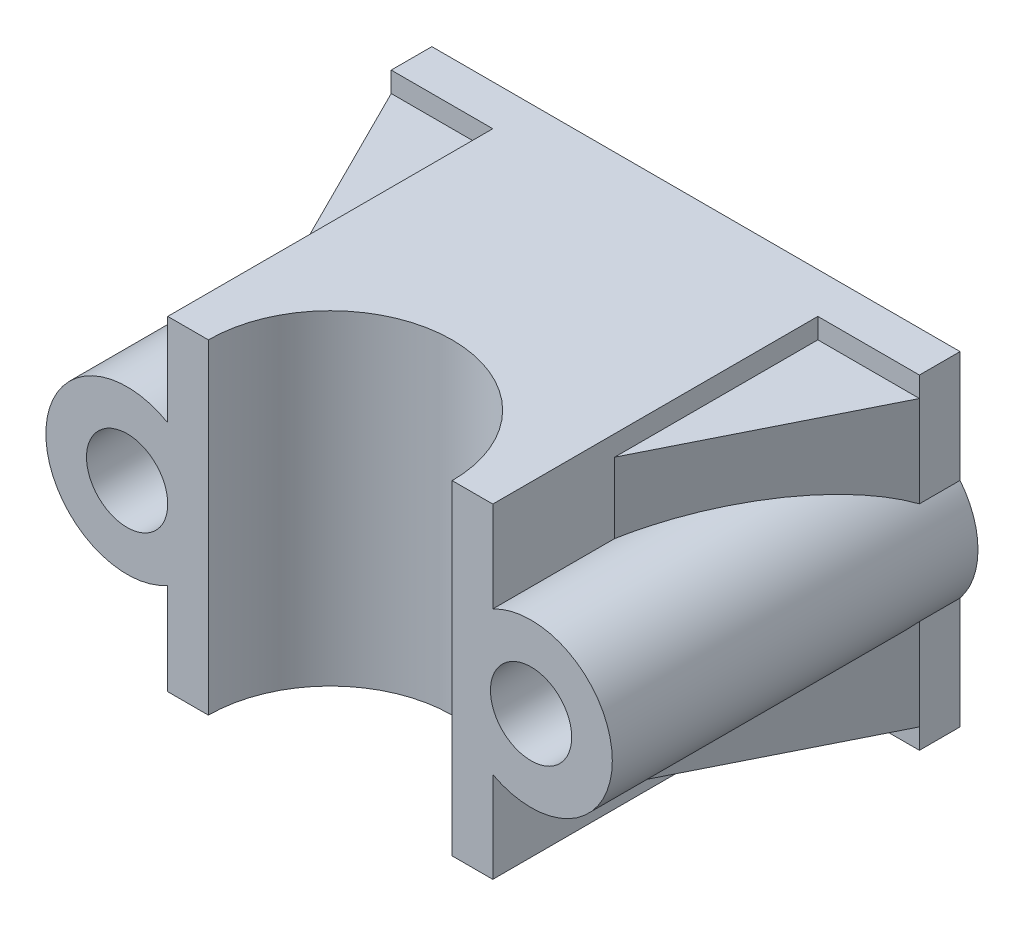
ISO-10303-21;
HEADER;
FILE_DESCRIPTION(('STEP AP214'),'2;1');
FILE_NAME('part.step','',(''),(''),'','','');
FILE_SCHEMA(('AUTOMOTIVE_DESIGN { 1 0 10303 214 1 1 1 1 }'));
ENDSEC;
DATA;
#1=APPLICATION_CONTEXT('core data for automotive mechanical design processes');
#2=APPLICATION_PROTOCOL_DEFINITION('international standard','automotive_design',2000,#1);
#3=PRODUCT_CONTEXT('',#1,'mechanical');
#4=PRODUCT('Part','Part','',(#3));
#5=PRODUCT_RELATED_PRODUCT_CATEGORY('part','',(#4));
#6=PRODUCT_DEFINITION_FORMATION('','',#4);
#7=PRODUCT_DEFINITION_CONTEXT('part definition',#1,'design');
#8=PRODUCT_DEFINITION('design','',#6,#7);
#9=PRODUCT_DEFINITION_SHAPE('','',#8);
#10=(LENGTH_UNIT() NAMED_UNIT(*) SI_UNIT(.MILLI.,.METRE.));
#11=(NAMED_UNIT(*) PLANE_ANGLE_UNIT() SI_UNIT($,.RADIAN.));
#12=(NAMED_UNIT(*) SI_UNIT($,.STERADIAN.) SOLID_ANGLE_UNIT());
#13=UNCERTAINTY_MEASURE_WITH_UNIT(LENGTH_MEASURE(1.E-05),#10,'distance_accuracy_value','');
#14=(GEOMETRIC_REPRESENTATION_CONTEXT(3) GLOBAL_UNCERTAINTY_ASSIGNED_CONTEXT((#13)) GLOBAL_UNIT_ASSIGNED_CONTEXT((#10,
#11,#12)) REPRESENTATION_CONTEXT('',''));
#15=CARTESIAN_POINT('',(0.,0.,0.));
#16=DIRECTION('',(0.,0.,1.));
#17=DIRECTION('',(1.,0.,0.));
#18=AXIS2_PLACEMENT_3D('',#15,#16,#17);
#19=CARTESIAN_POINT('',(105.,52.,60.));
#20=DIRECTION('',(0.894427190999916,0.,0.447213595499958));
#21=DIRECTION('',(0.447213595499958,0.,-0.894427190999916));
#22=AXIS2_PLACEMENT_3D('',#19,#20,#21);
#23=PLANE('',#22);
#24=DIRECTION('',(0.,1.,0.));
#25=VECTOR('',#24,1.);
#26=CARTESIAN_POINT('',(130.,0.,10.));
#27=LINE('',#26,#25);
#28=CARTESIAN_POINT('',(130.,52.5387472375144,10.));
#29=VERTEX_POINT('',#28);
#30=CARTESIAN_POINT('',(130.,75.,10.));
#31=VERTEX_POINT('',#30);
#32=EDGE_CURVE('E316',#29,#31,#27,.T.);
#33=ORIENTED_EDGE('',*,*,#32,.T.);
#34=DIRECTION('',(0.447213595499958,0.,-0.894427190999916));
#35=VECTOR('',#34,1.);
#36=CARTESIAN_POINT('',(130.,75.,10.));
#37=LINE('',#36,#35);
#38=CARTESIAN_POINT('',(105.,75.,60.));
#39=VERTEX_POINT('',#38);
#40=EDGE_CURVE('E420',#39,#31,#37,.T.);
#41=ORIENTED_EDGE('',*,*,#40,.F.);
#42=DIRECTION('',(0.,1.,0.));
#43=VECTOR('',#42,1.);
#44=CARTESIAN_POINT('',(105.,52.,60.));
#45=LINE('',#44,#43);
#46=CARTESIAN_POINT('',(105.,57.6434080653318,60.));
#47=VERTEX_POINT('',#46);
#48=EDGE_CURVE('E227',#47,#39,#45,.T.);
#49=ORIENTED_EDGE('',*,*,#48,.F.);
#50=CARTESIAN_POINT('',(114.418606682529,40.,41.1627866349416));
#51=DIRECTION('',(0.894427190999916,0.,0.447213595499958));
#52=DIRECTION('',(-0.447213595499958,0.,0.894427190999916));
#53=AXIS2_PLACEMENT_3D('',#50,#51,#52);
#54=ELLIPSE('',#53,44.7213595499958,20.);
#55=EDGE_CURVE('E54',#47,#29,#54,.F.);
#56=ORIENTED_EDGE('',*,*,#55,.T.);
#57=EDGE_LOOP('',(#33,#41,#49,#56));
#58=FACE_BOUND('',#57,.T.);
#59=ADVANCED_FACE('F50',(#58),#23,.T.);
#60=CARTESIAN_POINT('',(25.,28.,60.));
#61=DIRECTION('',(-0.894427190999916,0.,0.447213595499958));
#62=DIRECTION('',(0.447213595499958,0.,0.894427190999916));
#63=AXIS2_PLACEMENT_3D('',#60,#61,#62);
#64=PLANE('',#63);
#65=DIRECTION('',(0.,-1.,0.));
#66=VECTOR('',#65,1.);
#67=CARTESIAN_POINT('',(0.,80.,10.));
#68=LINE('',#67,#66);
#69=CARTESIAN_POINT('',(0.,26.771243444677,10.));
#70=VERTEX_POINT('',#69);
#71=CARTESIAN_POINT('',(0.,5.,10.));
#72=VERTEX_POINT('',#71);
#73=EDGE_CURVE('E324',#70,#72,#68,.T.);
#74=ORIENTED_EDGE('',*,*,#73,.T.);
#75=DIRECTION('',(-0.447213595499958,0.,-0.894427190999916));
#76=VECTOR('',#75,1.);
#77=CARTESIAN_POINT('',(0.,5.,10.));
#78=LINE('',#77,#76);
#79=CARTESIAN_POINT('',(25.,5.,60.));
#80=VERTEX_POINT('',#79);
#81=EDGE_CURVE('E426',#80,#72,#78,.T.);
#82=ORIENTED_EDGE('',*,*,#81,.F.);
#83=DIRECTION('',(0.,-1.,0.));
#84=VECTOR('',#83,1.);
#85=CARTESIAN_POINT('',(25.,28.,60.));
#86=LINE('',#85,#84);
#87=CARTESIAN_POINT('',(25.,22.6794919243112,60.));
#88=VERTEX_POINT('',#87);
#89=EDGE_CURVE('E233',#88,#80,#86,.T.);
#90=ORIENTED_EDGE('',*,*,#89,.F.);
#91=CARTESIAN_POINT('',(15.,40.,40.));
#92=DIRECTION('',(-0.894427190999916,0.,0.447213595499958));
#93=DIRECTION('',(0.447213595499958,0.,0.894427190999916));
#94=AXIS2_PLACEMENT_3D('',#91,#92,#93);
#95=ELLIPSE('',#94,44.7213595499958,20.);
#96=EDGE_CURVE('E359',#88,#70,#95,.F.);
#97=ORIENTED_EDGE('',*,*,#96,.T.);
#98=EDGE_LOOP('',(#74,#82,#90,#97));
#99=FACE_BOUND('',#98,.T.);
#100=ADVANCED_FACE('F466',(#99),#64,.T.);
#101=CARTESIAN_POINT('',(0.,80.,10.));
#102=DIRECTION('',(1.,0.,0.));
#103=DIRECTION('',(0.,0.,-1.));
#104=AXIS2_PLACEMENT_3D('',#101,#102,#103);
#105=PLANE('',#104);
#106=DIRECTION('',(0.,-1.,0.));
#107=VECTOR('',#106,1.);
#108=CARTESIAN_POINT('',(0.,80.,0.));
#109=LINE('',#108,#107);
#110=CARTESIAN_POINT('',(0.,80.,0.));
#111=VERTEX_POINT('',#110);
#112=CARTESIAN_POINT('',(0.,53.228756555323,0.));
#113=VERTEX_POINT('',#112);
#114=EDGE_CURVE('E326',#111,#113,#109,.T.);
#115=ORIENTED_EDGE('',*,*,#114,.T.);
#116=DIRECTION('',(0.,0.,1.));
#117=VECTOR('',#116,1.);
#118=CARTESIAN_POINT('',(0.,53.228756555323,0.));
#119=LINE('',#118,#117);
#120=CARTESIAN_POINT('',(0.,53.228756555323,10.));
#121=VERTEX_POINT('',#120);
#122=EDGE_CURVE('E263',#113,#121,#119,.T.);
#123=ORIENTED_EDGE('',*,*,#122,.T.);
#124=CARTESIAN_POINT('',(0.,75.,10.));
#125=VERTEX_POINT('',#124);
#126=EDGE_CURVE('E318',#125,#121,#68,.T.);
#127=ORIENTED_EDGE('',*,*,#126,.F.);
#128=CARTESIAN_POINT('',(0.,80.,10.));
#129=VERTEX_POINT('',#128);
#130=EDGE_CURVE('E320',#129,#125,#68,.T.);
#131=ORIENTED_EDGE('',*,*,#130,.F.);
#132=DIRECTION('',(0.,0.,-1.));
#133=VECTOR('',#132,1.);
#134=CARTESIAN_POINT('',(0.,80.,10.));
#135=LINE('',#134,#133);
#136=EDGE_CURVE('E322',#129,#111,#135,.T.);
#137=ORIENTED_EDGE('',*,*,#136,.T.);
#138=EDGE_LOOP('',(#115,#123,#127,#131,#137));
#139=FACE_BOUND('',#138,.T.);
#140=ADVANCED_FACE('F475',(#139),#105,.F.);
#141=CARTESIAN_POINT('',(25.,80.,0.));
#142=DIRECTION('',(1.,0.,0.));
#143=DIRECTION('',(0.,0.,-1.));
#144=AXIS2_PLACEMENT_3D('',#141,#142,#143);
#145=PLANE('',#144);
#146=DIRECTION('',(0.,0.,1.));
#147=VECTOR('',#146,1.);
#148=CARTESIAN_POINT('',(25.,80.,0.));
#149=LINE('',#148,#147);
#150=CARTESIAN_POINT('',(25.,80.,9.99999999999995));
#151=VERTEX_POINT('',#150);
#152=CARTESIAN_POINT('',(25.,80.,90.));
#153=VERTEX_POINT('',#152);
#154=EDGE_CURVE('E281',#151,#153,#149,.T.);
#155=ORIENTED_EDGE('',*,*,#154,.F.);
#156=DIRECTION('',(0.,1.,0.));
#157=VECTOR('',#156,1.);
#158=CARTESIAN_POINT('',(25.,75.,9.99999999999995));
#159=LINE('',#158,#157);
#160=CARTESIAN_POINT('',(25.,75.,9.99999999999995));
#161=VERTEX_POINT('',#160);
#162=EDGE_CURVE('E219',#161,#151,#159,.T.);
#163=ORIENTED_EDGE('',*,*,#162,.F.);
#164=DIRECTION('',(0.,0.,-1.));
#165=VECTOR('',#164,1.);
#166=CARTESIAN_POINT('',(25.,75.,59.9999999999999));
#167=LINE('',#166,#165);
#168=CARTESIAN_POINT('',(25.,75.,59.9999999999999));
#169=VERTEX_POINT('',#168);
#170=EDGE_CURVE('E214',#169,#161,#167,.T.);
#171=ORIENTED_EDGE('',*,*,#170,.F.);
#172=DIRECTION('',(0.,1.,0.));
#173=VECTOR('',#172,1.);
#174=CARTESIAN_POINT('',(25.,52.,60.));
#175=LINE('',#174,#173);
#176=CARTESIAN_POINT('',(25.,57.3205080756888,60.));
#177=VERTEX_POINT('',#176);
#178=EDGE_CURVE('E213',#177,#169,#175,.T.);
#179=ORIENTED_EDGE('',*,*,#178,.F.);
#180=DIRECTION('',(0.,0.,1.));
#181=VECTOR('',#180,1.);
#182=CARTESIAN_POINT('',(25.,57.3205080756888,0.));
#183=LINE('',#182,#181);
#184=CARTESIAN_POINT('',(25.,57.3205080756888,90.));
#185=VERTEX_POINT('',#184);
#186=EDGE_CURVE('E354',#177,#185,#183,.T.);
#187=ORIENTED_EDGE('',*,*,#186,.T.);
#188=DIRECTION('',(0.,-1.,0.));
#189=VECTOR('',#188,1.);
#190=CARTESIAN_POINT('',(25.,80.,90.));
#191=LINE('',#190,#189);
#192=EDGE_CURVE('E313',#153,#185,#191,.T.);
#193=ORIENTED_EDGE('',*,*,#192,.F.);
#194=EDGE_LOOP('',(#155,#163,#171,#179,#187,#193));
#195=FACE_BOUND('',#194,.T.);
#196=ADVANCED_FACE('F211',(#195),#145,.F.);
#197=CARTESIAN_POINT('',(130.,0.,10.));
#198=DIRECTION('',(-1.,0.,0.));
#199=DIRECTION('',(0.,0.,1.));
#200=AXIS2_PLACEMENT_3D('',#197,#198,#199);
#201=PLANE('',#200);
#202=DIRECTION('',(0.,1.,0.));
#203=VECTOR('',#202,1.);
#204=CARTESIAN_POINT('',(130.,0.,0.));
#205=LINE('',#204,#203);
#206=CARTESIAN_POINT('',(130.,0.,0.));
#207=VERTEX_POINT('',#206);
#208=CARTESIAN_POINT('',(130.,27.4612527624856,0.));
#209=VERTEX_POINT('',#208);
#210=EDGE_CURVE('E331',#207,#209,#205,.T.);
#211=ORIENTED_EDGE('',*,*,#210,.T.);
#212=DIRECTION('',(0.,0.,1.));
#213=VECTOR('',#212,1.);
#214=CARTESIAN_POINT('',(130.,27.4612527624856,0.));
#215=LINE('',#214,#213);
#216=CARTESIAN_POINT('',(130.,27.4612527624856,10.));
#217=VERTEX_POINT('',#216);
#218=EDGE_CURVE('E273',#209,#217,#215,.T.);
#219=ORIENTED_EDGE('',*,*,#218,.T.);
#220=CARTESIAN_POINT('',(130.,5.,10.));
#221=VERTEX_POINT('',#220);
#222=EDGE_CURVE('E329',#221,#217,#27,.T.);
#223=ORIENTED_EDGE('',*,*,#222,.F.);
#224=CARTESIAN_POINT('',(130.,0.,10.));
#225=VERTEX_POINT('',#224);
#226=EDGE_CURVE('E321',#225,#221,#27,.T.);
#227=ORIENTED_EDGE('',*,*,#226,.F.);
#228=DIRECTION('',(0.,0.,-1.));
#229=VECTOR('',#228,1.);
#230=CARTESIAN_POINT('',(130.,0.,10.));
#231=LINE('',#230,#229);
#232=EDGE_CURVE('E341',#225,#207,#231,.T.);
#233=ORIENTED_EDGE('',*,*,#232,.T.);
#234=EDGE_LOOP('',(#211,#219,#223,#227,#233));
#235=FACE_BOUND('',#234,.T.);
#236=ADVANCED_FACE('F398',(#235),#201,.F.);
#237=CARTESIAN_POINT('',(105.,80.,0.));
#238=DIRECTION('',(1.,0.,0.));
#239=DIRECTION('',(0.,0.,-1.));
#240=AXIS2_PLACEMENT_3D('',#237,#238,#239);
#241=PLANE('',#240);
#242=ORIENTED_EDGE('',*,*,#48,.T.);
#243=DIRECTION('',(0.,0.,1.));
#244=VECTOR('',#243,1.);
#245=CARTESIAN_POINT('',(105.,75.,60.));
#246=LINE('',#245,#244);
#247=CARTESIAN_POINT('',(105.,75.,9.99999999999995));
#248=VERTEX_POINT('',#247);
#249=EDGE_CURVE('E61',#248,#39,#246,.T.);
#250=ORIENTED_EDGE('',*,*,#249,.F.);
#251=DIRECTION('',(0.,1.,0.));
#252=VECTOR('',#251,1.);
#253=CARTESIAN_POINT('',(105.,75.,9.99999999999995));
#254=LINE('',#253,#252);
#255=CARTESIAN_POINT('',(105.,80.,9.99999999999995));
#256=VERTEX_POINT('',#255);
#257=EDGE_CURVE('E425',#248,#256,#254,.T.);
#258=ORIENTED_EDGE('',*,*,#257,.T.);
#259=DIRECTION('',(0.,0.,1.));
#260=VECTOR('',#259,1.);
#261=CARTESIAN_POINT('',(105.,80.,0.));
#262=LINE('',#261,#260);
#263=CARTESIAN_POINT('',(105.,80.,90.));
#264=VERTEX_POINT('',#263);
#265=EDGE_CURVE('E282',#256,#264,#262,.T.);
#266=ORIENTED_EDGE('',*,*,#265,.T.);
#267=DIRECTION('',(0.,-1.,0.));
#268=VECTOR('',#267,1.);
#269=CARTESIAN_POINT('',(105.,80.,90.));
#270=LINE('',#269,#268);
#271=CARTESIAN_POINT('',(105.,57.6434080653318,90.));
#272=VERTEX_POINT('',#271);
#273=EDGE_CURVE('E309',#264,#272,#270,.T.);
#274=ORIENTED_EDGE('',*,*,#273,.T.);
#275=DIRECTION('',(0.,0.,1.));
#276=VECTOR('',#275,1.);
#277=CARTESIAN_POINT('',(105.,57.6434080653318,0.));
#278=LINE('',#277,#276);
#279=EDGE_CURVE('E347',#47,#272,#278,.T.);
#280=ORIENTED_EDGE('',*,*,#279,.F.);
#281=EDGE_LOOP('',(#242,#250,#258,#266,#274,#280));
#282=FACE_BOUND('',#281,.T.);
#283=ADVANCED_FACE('F375',(#282),#241,.T.);
#284=ORIENTED_EDGE('',*,*,#73,.F.);
#285=DIRECTION('',(0.,0.,1.));
#286=VECTOR('',#285,1.);
#287=CARTESIAN_POINT('',(0.,26.771243444677,0.));
#288=LINE('',#287,#286);
#289=CARTESIAN_POINT('',(0.,26.771243444677,0.));
#290=VERTEX_POINT('',#289);
#291=EDGE_CURVE('E257',#70,#290,#288,.F.);
#292=ORIENTED_EDGE('',*,*,#291,.T.);
#293=CARTESIAN_POINT('',(0.,0.,0.));
#294=VERTEX_POINT('',#293);
#295=EDGE_CURVE('E310',#290,#294,#109,.T.);
#296=ORIENTED_EDGE('',*,*,#295,.T.);
#297=DIRECTION('',(0.,0.,-1.));
#298=VECTOR('',#297,1.);
#299=CARTESIAN_POINT('',(0.,0.,10.));
#300=LINE('',#299,#298);
#301=CARTESIAN_POINT('',(0.,0.,10.));
#302=VERTEX_POINT('',#301);
#303=EDGE_CURVE('E342',#302,#294,#300,.T.);
#304=ORIENTED_EDGE('',*,*,#303,.F.);
#305=DIRECTION('',(0.,-1.,0.));
#306=VECTOR('',#305,1.);
#307=CARTESIAN_POINT('',(0.,5.,10.));
#308=LINE('',#307,#306);
#309=EDGE_CURVE('E234',#72,#302,#308,.T.);
#310=ORIENTED_EDGE('',*,*,#309,.F.);
#311=EDGE_LOOP('',(#284,#292,#296,#304,#310));
#312=FACE_BOUND('',#311,.T.);
#313=ADVANCED_FACE('F47',(#312),#105,.F.);
#314=CARTESIAN_POINT('',(0.,0.,10.));
#315=DIRECTION('',(0.,1.,0.));
#316=DIRECTION('',(0.,0.,1.));
#317=AXIS2_PLACEMENT_3D('',#314,#315,#316);
#318=PLANE('',#317);
#319=DIRECTION('',(0.,0.,1.));
#320=VECTOR('',#319,1.);
#321=CARTESIAN_POINT('',(25.,0.,0.));
#322=LINE('',#321,#320);
#323=CARTESIAN_POINT('',(25.,0.,9.99999999999999));
#324=VERTEX_POINT('',#323);
#325=CARTESIAN_POINT('',(25.,0.,90.));
#326=VERTEX_POINT('',#325);
#327=EDGE_CURVE('E294',#324,#326,#322,.T.);
#328=ORIENTED_EDGE('',*,*,#327,.F.);
#329=DIRECTION('',(1.,0.,0.));
#330=VECTOR('',#329,1.);
#331=CARTESIAN_POINT('',(25.,0.,9.99999999999999));
#332=LINE('',#331,#330);
#333=EDGE_CURVE('E435',#302,#324,#332,.T.);
#334=ORIENTED_EDGE('',*,*,#333,.F.);
#335=ORIENTED_EDGE('',*,*,#303,.T.);
#336=DIRECTION('',(1.,0.,0.));
#337=VECTOR('',#336,1.);
#338=CARTESIAN_POINT('',(0.,0.,0.));
#339=LINE('',#338,#337);
#340=EDGE_CURVE('E327',#294,#207,#339,.T.);
#341=ORIENTED_EDGE('',*,*,#340,.T.);
#342=ORIENTED_EDGE('',*,*,#232,.F.);
#343=DIRECTION('',(1.,0.,0.));
#344=VECTOR('',#343,1.);
#345=CARTESIAN_POINT('',(105.,0.,9.99999999999999));
#346=LINE('',#345,#344);
#347=CARTESIAN_POINT('',(105.,0.,9.99999999999999));
#348=VERTEX_POINT('',#347);
#349=EDGE_CURVE('E441',#348,#225,#346,.T.);
#350=ORIENTED_EDGE('',*,*,#349,.F.);
#351=DIRECTION('',(0.,0.,1.));
#352=VECTOR('',#351,1.);
#353=CARTESIAN_POINT('',(105.,0.,0.));
#354=LINE('',#353,#352);
#355=CARTESIAN_POINT('',(105.,0.,90.));
#356=VERTEX_POINT('',#355);
#357=EDGE_CURVE('E300',#348,#356,#354,.T.);
#358=ORIENTED_EDGE('',*,*,#357,.T.);
#359=DIRECTION('',(-1.,0.,0.));
#360=VECTOR('',#359,1.);
#361=CARTESIAN_POINT('',(0.,0.,90.));
#362=LINE('',#361,#360);
#363=CARTESIAN_POINT('',(95.,0.,90.));
#364=VERTEX_POINT('',#363);
#365=EDGE_CURVE('E299',#356,#364,#362,.T.);
#366=ORIENTED_EDGE('',*,*,#365,.T.);
#367=CARTESIAN_POINT('',(65.,0.,90.));
#368=DIRECTION('',(0.,-1.,0.));
#369=DIRECTION('',(0.,0.,-1.));
#370=AXIS2_PLACEMENT_3D('',#367,#368,#369);
#371=CIRCLE('',#370,30.);
#372=CARTESIAN_POINT('',(35.,0.,90.));
#373=VERTEX_POINT('',#372);
#374=EDGE_CURVE('E285',#373,#364,#371,.T.);
#375=ORIENTED_EDGE('',*,*,#374,.F.);
#376=DIRECTION('',(1.,0.,0.));
#377=VECTOR('',#376,1.);
#378=CARTESIAN_POINT('',(0.,0.,90.));
#379=LINE('',#378,#377);
#380=EDGE_CURVE('E280',#326,#373,#379,.T.);
#381=ORIENTED_EDGE('',*,*,#380,.F.);
#382=EDGE_LOOP('',(#328,#334,#335,#341,#342,#350,#358,#366,#375,#381));
#383=FACE_BOUND('',#382,.T.);
#384=ADVANCED_FACE('F520',(#383),#318,.F.);
#385=ORIENTED_EDGE('',*,*,#32,.F.);
#386=DIRECTION('',(0.,0.,1.));
#387=VECTOR('',#386,1.);
#388=CARTESIAN_POINT('',(130.,52.5387472375144,0.));
#389=LINE('',#388,#387);
#390=CARTESIAN_POINT('',(130.,52.5387472375144,0.));
#391=VERTEX_POINT('',#390);
#392=EDGE_CURVE('E272',#29,#391,#389,.F.);
#393=ORIENTED_EDGE('',*,*,#392,.T.);
#394=CARTESIAN_POINT('',(130.,80.,0.));
#395=VERTEX_POINT('',#394);
#396=EDGE_CURVE('E335',#391,#395,#205,.T.);
#397=ORIENTED_EDGE('',*,*,#396,.T.);
#398=DIRECTION('',(0.,0.,-1.));
#399=VECTOR('',#398,1.);
#400=CARTESIAN_POINT('',(130.,80.,10.));
#401=LINE('',#400,#399);
#402=CARTESIAN_POINT('',(130.,80.,10.));
#403=VERTEX_POINT('',#402);
#404=EDGE_CURVE('E339',#403,#395,#401,.T.);
#405=ORIENTED_EDGE('',*,*,#404,.F.);
#406=DIRECTION('',(0.,1.,0.));
#407=VECTOR('',#406,1.);
#408=CARTESIAN_POINT('',(130.,75.,10.));
#409=LINE('',#408,#407);
#410=EDGE_CURVE('E428',#31,#403,#409,.T.);
#411=ORIENTED_EDGE('',*,*,#410,.F.);
#412=EDGE_LOOP('',(#385,#393,#397,#405,#411));
#413=FACE_BOUND('',#412,.T.);
#414=ADVANCED_FACE('F410',(#413),#201,.F.);
#415=CARTESIAN_POINT('',(130.,80.,10.));
#416=DIRECTION('',(0.,-1.,0.));
#417=DIRECTION('',(0.,0.,-1.));
#418=AXIS2_PLACEMENT_3D('',#415,#416,#417);
#419=PLANE('',#418);
#420=ORIENTED_EDGE('',*,*,#136,.F.);
#421=DIRECTION('',(-1.,0.,0.));
#422=VECTOR('',#421,1.);
#423=CARTESIAN_POINT('',(25.,80.,9.99999999999995));
#424=LINE('',#423,#422);
#425=EDGE_CURVE('E221',#151,#129,#424,.T.);
#426=ORIENTED_EDGE('',*,*,#425,.F.);
#427=ORIENTED_EDGE('',*,*,#154,.T.);
#428=DIRECTION('',(1.,0.,0.));
#429=VECTOR('',#428,1.);
#430=CARTESIAN_POINT('',(0.,80.,90.));
#431=LINE('',#430,#429);
#432=CARTESIAN_POINT('',(35.,80.,90.));
#433=VERTEX_POINT('',#432);
#434=EDGE_CURVE('E278',#153,#433,#431,.T.);
#435=ORIENTED_EDGE('',*,*,#434,.T.);
#436=CARTESIAN_POINT('',(65.,80.,90.));
#437=DIRECTION('',(0.,-1.,0.));
#438=DIRECTION('',(0.,0.,-1.));
#439=AXIS2_PLACEMENT_3D('',#436,#437,#438);
#440=CIRCLE('',#439,30.);
#441=CARTESIAN_POINT('',(95.,80.,90.));
#442=VERTEX_POINT('',#441);
#443=EDGE_CURVE('E289',#433,#442,#440,.T.);
#444=ORIENTED_EDGE('',*,*,#443,.T.);
#445=DIRECTION('',(-1.,0.,0.));
#446=VECTOR('',#445,1.);
#447=CARTESIAN_POINT('',(0.,80.,90.));
#448=LINE('',#447,#446);
#449=EDGE_CURVE('E290',#264,#442,#448,.T.);
#450=ORIENTED_EDGE('',*,*,#449,.F.);
#451=ORIENTED_EDGE('',*,*,#265,.F.);
#452=DIRECTION('',(-1.,0.,0.));
#453=VECTOR('',#452,1.);
#454=CARTESIAN_POINT('',(105.,80.,9.99999999999995));
#455=LINE('',#454,#453);
#456=EDGE_CURVE('E412',#403,#256,#455,.T.);
#457=ORIENTED_EDGE('',*,*,#456,.F.);
#458=ORIENTED_EDGE('',*,*,#404,.T.);
#459=DIRECTION('',(-1.,0.,0.));
#460=VECTOR('',#459,1.);
#461=CARTESIAN_POINT('',(130.,80.,0.));
#462=LINE('',#461,#460);
#463=EDGE_CURVE('E334',#395,#111,#462,.T.);
#464=ORIENTED_EDGE('',*,*,#463,.T.);
#465=EDGE_LOOP('',(#420,#426,#427,#435,#444,#450,#451,#457,#458,#464));
#466=FACE_BOUND('',#465,.T.);
#467=ADVANCED_FACE('F415',(#466),#419,.F.);
#468=CARTESIAN_POINT('',(0.,0.,0.));
#469=DIRECTION('',(0.,0.,1.));
#470=DIRECTION('',(1.,0.,0.));
#471=AXIS2_PLACEMENT_3D('',#468,#469,#470);
#472=PLANE('',#471);
#473=CARTESIAN_POINT('',(114.418606682529,40.,0.));
#474=DIRECTION('',(0.,0.,1.));
#475=DIRECTION('',(1.,0.,0.));
#476=AXIS2_PLACEMENT_3D('',#473,#474,#475);
#477=CIRCLE('',#476,10.);
#478=CARTESIAN_POINT('',(124.418606682529,40.,0.));
#479=VERTEX_POINT('',#478);
#480=EDGE_CURVE('E246',#479,#479,#477,.T.);
#481=ORIENTED_EDGE('',*,*,#480,.T.);
#482=EDGE_LOOP('',(#481));
#483=FACE_BOUND('',#482,.T.);
#484=CARTESIAN_POINT('',(15.,40.,0.));
#485=DIRECTION('',(0.,0.,1.));
#486=DIRECTION('',(1.,0.,0.));
#487=AXIS2_PLACEMENT_3D('',#484,#485,#486);
#488=CIRCLE('',#487,10.);
#489=CARTESIAN_POINT('',(25.,40.,0.));
#490=VERTEX_POINT('',#489);
#491=EDGE_CURVE('E254',#490,#490,#488,.T.);
#492=ORIENTED_EDGE('',*,*,#491,.T.);
#493=EDGE_LOOP('',(#492));
#494=FACE_BOUND('',#493,.T.);
#495=ORIENTED_EDGE('',*,*,#295,.F.);
#496=CARTESIAN_POINT('',(15.,40.,0.));
#497=DIRECTION('',(0.,0.,1.));
#498=DIRECTION('',(1.,0.,0.));
#499=AXIS2_PLACEMENT_3D('',#496,#497,#498);
#500=CIRCLE('',#499,20.);
#501=EDGE_CURVE('E260',#113,#290,#500,.T.);
#502=ORIENTED_EDGE('',*,*,#501,.F.);
#503=ORIENTED_EDGE('',*,*,#114,.F.);
#504=ORIENTED_EDGE('',*,*,#463,.F.);
#505=ORIENTED_EDGE('',*,*,#396,.F.);
#506=CARTESIAN_POINT('',(114.418606682529,40.,0.));
#507=DIRECTION('',(0.,0.,1.));
#508=DIRECTION('',(1.,0.,0.));
#509=AXIS2_PLACEMENT_3D('',#506,#507,#508);
#510=CIRCLE('',#509,20.);
#511=EDGE_CURVE('E266',#209,#391,#510,.T.);
#512=ORIENTED_EDGE('',*,*,#511,.F.);
#513=ORIENTED_EDGE('',*,*,#210,.F.);
#514=ORIENTED_EDGE('',*,*,#340,.F.);
#515=EDGE_LOOP('',(#495,#502,#503,#504,#505,#512,#513,#514));
#516=FACE_BOUND('',#515,.T.);
#517=ADVANCED_FACE('F405',(#483,#494,#516),#472,.F.);
#518=CARTESIAN_POINT('',(0.,80.,90.));
#519=DIRECTION('',(0.,0.,-1.));
#520=DIRECTION('',(-1.,0.,0.));
#521=AXIS2_PLACEMENT_3D('',#518,#519,#520);
#522=PLANE('',#521);
#523=CARTESIAN_POINT('',(15.,40.,90.));
#524=DIRECTION('',(0.,0.,1.));
#525=DIRECTION('',(1.,0.,0.));
#526=AXIS2_PLACEMENT_3D('',#523,#524,#525);
#527=CIRCLE('',#526,10.);
#528=CARTESIAN_POINT('',(25.,40.,90.));
#529=VERTEX_POINT('',#528);
#530=EDGE_CURVE('E244',#529,#529,#527,.T.);
#531=ORIENTED_EDGE('',*,*,#530,.F.);
#532=EDGE_LOOP('',(#531));
#533=FACE_BOUND('',#532,.T.);
#534=ORIENTED_EDGE('',*,*,#380,.T.);
#535=DIRECTION('',(0.,-1.,0.));
#536=VECTOR('',#535,1.);
#537=CARTESIAN_POINT('',(35.,80.,90.));
#538=LINE('',#537,#536);
#539=EDGE_CURVE('E302',#433,#373,#538,.T.);
#540=ORIENTED_EDGE('',*,*,#539,.F.);
#541=ORIENTED_EDGE('',*,*,#434,.F.);
#542=ORIENTED_EDGE('',*,*,#192,.T.);
#543=CARTESIAN_POINT('',(15.,40.,90.));
#544=DIRECTION('',(0.,0.,1.));
#545=DIRECTION('',(1.,0.,0.));
#546=AXIS2_PLACEMENT_3D('',#543,#544,#545);
#547=CIRCLE('',#546,20.);
#548=CARTESIAN_POINT('',(25.,22.6794919243112,90.));
#549=VERTEX_POINT('',#548);
#550=EDGE_CURVE('E248',#185,#549,#547,.T.);
#551=ORIENTED_EDGE('',*,*,#550,.T.);
#552=EDGE_CURVE('E292',#549,#326,#191,.T.);
#553=ORIENTED_EDGE('',*,*,#552,.T.);
#554=EDGE_LOOP('',(#534,#540,#541,#542,#551,#553));
#555=FACE_BOUND('',#554,.T.);
#556=ADVANCED_FACE('F497',(#533,#555),#522,.F.);
#557=CARTESIAN_POINT('',(65.,80.,90.));
#558=DIRECTION('',(0.,-1.,0.));
#559=DIRECTION('',(0.,0.,-1.));
#560=AXIS2_PLACEMENT_3D('',#557,#558,#559);
#561=CYLINDRICAL_SURFACE('',#560,30.);
#562=ORIENTED_EDGE('',*,*,#374,.T.);
#563=DIRECTION('',(0.,-1.,0.));
#564=VECTOR('',#563,1.);
#565=CARTESIAN_POINT('',(95.,80.,90.));
#566=LINE('',#565,#564);
#567=EDGE_CURVE('E308',#442,#364,#566,.T.);
#568=ORIENTED_EDGE('',*,*,#567,.F.);
#569=ORIENTED_EDGE('',*,*,#443,.F.);
#570=ORIENTED_EDGE('',*,*,#539,.T.);
#571=EDGE_LOOP('',(#562,#568,#569,#570));
#572=FACE_BOUND('',#571,.T.);
#573=ADVANCED_FACE('F496',(#572),#561,.F.);
#574=CARTESIAN_POINT('',(0.,80.,90.));
#575=DIRECTION('',(0.,0.,1.));
#576=DIRECTION('',(1.,0.,0.));
#577=AXIS2_PLACEMENT_3D('',#574,#575,#576);
#578=PLANE('',#577);
#579=CARTESIAN_POINT('',(114.418606682529,40.,90.));
#580=DIRECTION('',(0.,0.,1.));
#581=DIRECTION('',(1.,0.,0.));
#582=AXIS2_PLACEMENT_3D('',#579,#580,#581);
#583=CIRCLE('',#582,10.);
#584=CARTESIAN_POINT('',(124.418606682529,40.,90.));
#585=VERTEX_POINT('',#584);
#586=EDGE_CURVE('E249',#585,#585,#583,.T.);
#587=ORIENTED_EDGE('',*,*,#586,.F.);
#588=EDGE_LOOP('',(#587));
#589=FACE_BOUND('',#588,.T.);
#590=ORIENTED_EDGE('',*,*,#365,.F.);
#591=CARTESIAN_POINT('',(105.,22.3565919346682,90.));
#592=VERTEX_POINT('',#591);
#593=EDGE_CURVE('E312',#592,#356,#270,.T.);
#594=ORIENTED_EDGE('',*,*,#593,.F.);
#595=CARTESIAN_POINT('',(114.418606682529,40.,90.));
#596=DIRECTION('',(0.,0.,1.));
#597=DIRECTION('',(1.,0.,0.));
#598=AXIS2_PLACEMENT_3D('',#595,#596,#597);
#599=CIRCLE('',#598,20.);
#600=EDGE_CURVE('E270',#592,#272,#599,.T.);
#601=ORIENTED_EDGE('',*,*,#600,.T.);
#602=ORIENTED_EDGE('',*,*,#273,.F.);
#603=ORIENTED_EDGE('',*,*,#449,.T.);
#604=ORIENTED_EDGE('',*,*,#567,.T.);
#605=EDGE_LOOP('',(#590,#594,#601,#602,#603,#604));
#606=FACE_BOUND('',#605,.T.);
#607=ADVANCED_FACE('F377',(#589,#606),#578,.T.);
#608=DIRECTION('',(0.,-1.,0.));
#609=VECTOR('',#608,1.);
#610=CARTESIAN_POINT('',(105.,28.,60.));
#611=LINE('',#610,#609);
#612=CARTESIAN_POINT('',(105.,22.3565919346682,60.));
#613=VERTEX_POINT('',#612);
#614=CARTESIAN_POINT('',(105.,5.,60.));
#615=VERTEX_POINT('',#614);
#616=EDGE_CURVE('E245',#613,#615,#611,.T.);
#617=ORIENTED_EDGE('',*,*,#616,.F.);
#618=DIRECTION('',(0.,0.,1.));
#619=VECTOR('',#618,1.);
#620=CARTESIAN_POINT('',(105.,22.3565919346682,0.));
#621=LINE('',#620,#619);
#622=EDGE_CURVE('E350',#592,#613,#621,.F.);
#623=ORIENTED_EDGE('',*,*,#622,.F.);
#624=ORIENTED_EDGE('',*,*,#593,.T.);
#625=ORIENTED_EDGE('',*,*,#357,.F.);
#626=DIRECTION('',(0.,-1.,0.));
#627=VECTOR('',#626,1.);
#628=CARTESIAN_POINT('',(105.,5.,9.99999999999999));
#629=LINE('',#628,#627);
#630=CARTESIAN_POINT('',(105.,5.,9.99999999999999));
#631=VERTEX_POINT('',#630);
#632=EDGE_CURVE('E240',#631,#348,#629,.T.);
#633=ORIENTED_EDGE('',*,*,#632,.F.);
#634=DIRECTION('',(0.,0.,-1.));
#635=VECTOR('',#634,1.);
#636=CARTESIAN_POINT('',(105.,5.,60.));
#637=LINE('',#636,#635);
#638=EDGE_CURVE('E386',#615,#631,#637,.T.);
#639=ORIENTED_EDGE('',*,*,#638,.F.);
#640=EDGE_LOOP('',(#617,#623,#624,#625,#633,#639));
#641=FACE_BOUND('',#640,.T.);
#642=ADVANCED_FACE('F383',(#641),#241,.T.);
#643=DIRECTION('',(0.,0.,1.));
#644=VECTOR('',#643,1.);
#645=CARTESIAN_POINT('',(25.,22.6794919243112,0.));
#646=LINE('',#645,#644);
#647=EDGE_CURVE('E355',#549,#88,#646,.F.);
#648=ORIENTED_EDGE('',*,*,#647,.T.);
#649=ORIENTED_EDGE('',*,*,#89,.T.);
#650=DIRECTION('',(0.,0.,1.));
#651=VECTOR('',#650,1.);
#652=CARTESIAN_POINT('',(25.,5.,60.));
#653=LINE('',#652,#651);
#654=CARTESIAN_POINT('',(25.,5.,9.99999999999999));
#655=VERTEX_POINT('',#654);
#656=EDGE_CURVE('E434',#655,#80,#653,.T.);
#657=ORIENTED_EDGE('',*,*,#656,.F.);
#658=DIRECTION('',(0.,-1.,0.));
#659=VECTOR('',#658,1.);
#660=CARTESIAN_POINT('',(25.,5.,9.99999999999999));
#661=LINE('',#660,#659);
#662=EDGE_CURVE('E226',#655,#324,#661,.T.);
#663=ORIENTED_EDGE('',*,*,#662,.T.);
#664=ORIENTED_EDGE('',*,*,#327,.T.);
#665=ORIENTED_EDGE('',*,*,#552,.F.);
#666=EDGE_LOOP('',(#648,#649,#657,#663,#664,#665));
#667=FACE_BOUND('',#666,.T.);
#668=ADVANCED_FACE('F492',(#667),#145,.F.);
#669=CARTESIAN_POINT('',(114.418606682529,40.,0.));
#670=DIRECTION('',(0.,0.,1.));
#671=DIRECTION('',(1.,0.,0.));
#672=AXIS2_PLACEMENT_3D('',#669,#670,#671);
#673=CYLINDRICAL_SURFACE('',#672,20.);
#674=ORIENTED_EDGE('',*,*,#55,.F.);
#675=ORIENTED_EDGE('',*,*,#279,.T.);
#676=ORIENTED_EDGE('',*,*,#600,.F.);
#677=ORIENTED_EDGE('',*,*,#622,.T.);
#678=CARTESIAN_POINT('',(114.418606682529,40.,41.1627866349416));
#679=DIRECTION('',(0.894427190999916,0.,0.447213595499958));
#680=DIRECTION('',(-0.447213595499958,0.,0.894427190999916));
#681=AXIS2_PLACEMENT_3D('',#678,#679,#680);
#682=ELLIPSE('',#681,44.7213595499958,20.);
#683=EDGE_CURVE('E357',#217,#613,#682,.F.);
#684=ORIENTED_EDGE('',*,*,#683,.F.);
#685=ORIENTED_EDGE('',*,*,#218,.F.);
#686=ORIENTED_EDGE('',*,*,#511,.T.);
#687=ORIENTED_EDGE('',*,*,#392,.F.);
#688=EDGE_LOOP('',(#674,#675,#676,#677,#684,#685,#686,#687));
#689=FACE_BOUND('',#688,.T.);
#690=ADVANCED_FACE('F367',(#689),#673,.T.);
#691=CARTESIAN_POINT('',(15.,40.,0.));
#692=DIRECTION('',(0.,0.,1.));
#693=DIRECTION('',(1.,0.,0.));
#694=AXIS2_PLACEMENT_3D('',#691,#692,#693);
#695=CYLINDRICAL_SURFACE('',#694,20.);
#696=CARTESIAN_POINT('',(15.,40.,40.));
#697=DIRECTION('',(-0.894427190999916,0.,0.447213595499958));
#698=DIRECTION('',(0.447213595499958,0.,0.894427190999916));
#699=AXIS2_PLACEMENT_3D('',#696,#697,#698);
#700=ELLIPSE('',#699,44.7213595499958,20.);
#701=EDGE_CURVE('E11',#121,#177,#700,.F.);
#702=ORIENTED_EDGE('',*,*,#701,.F.);
#703=ORIENTED_EDGE('',*,*,#122,.F.);
#704=ORIENTED_EDGE('',*,*,#501,.T.);
#705=ORIENTED_EDGE('',*,*,#291,.F.);
#706=ORIENTED_EDGE('',*,*,#96,.F.);
#707=ORIENTED_EDGE('',*,*,#647,.F.);
#708=ORIENTED_EDGE('',*,*,#550,.F.);
#709=ORIENTED_EDGE('',*,*,#186,.F.);
#710=EDGE_LOOP('',(#702,#703,#704,#705,#706,#707,#708,#709));
#711=FACE_BOUND('',#710,.T.);
#712=ADVANCED_FACE('F484',(#711),#695,.T.);
#713=CARTESIAN_POINT('',(114.418606682529,40.,0.));
#714=DIRECTION('',(0.,0.,1.));
#715=DIRECTION('',(1.,0.,0.));
#716=AXIS2_PLACEMENT_3D('',#713,#714,#715);
#717=CYLINDRICAL_SURFACE('',#716,10.);
#718=CARTESIAN_POINT('',(124.418606682529,40.,0.));
#719=CARTESIAN_POINT('',(124.418606682529,40.,0.937499999999998));
#720=CARTESIAN_POINT('',(124.418606682529,40.,1.875));
#721=CARTESIAN_POINT('',(124.418606682529,40.,3.75));
#722=CARTESIAN_POINT('',(124.418606682529,40.,4.6875));
#723=CARTESIAN_POINT('',(124.418606682529,40.,6.5625));
#724=CARTESIAN_POINT('',(124.418606682529,40.,7.5));
#725=CARTESIAN_POINT('',(124.418606682529,40.,9.375));
#726=CARTESIAN_POINT('',(124.418606682529,40.,10.3125));
#727=CARTESIAN_POINT('',(124.418606682529,40.,12.1875));
#728=CARTESIAN_POINT('',(124.418606682529,40.,13.125));
#729=CARTESIAN_POINT('',(124.418606682529,40.,15.));
#730=CARTESIAN_POINT('',(124.418606682529,40.,15.9375));
#731=CARTESIAN_POINT('',(124.418606682529,40.,17.8125));
#732=CARTESIAN_POINT('',(124.418606682529,40.,18.75));
#733=CARTESIAN_POINT('',(124.418606682529,40.,20.625));
#734=CARTESIAN_POINT('',(124.418606682529,40.,21.5625));
#735=CARTESIAN_POINT('',(124.418606682529,40.,23.4375));
#736=CARTESIAN_POINT('',(124.418606682529,40.,24.375));
#737=CARTESIAN_POINT('',(124.418606682529,40.,26.25));
#738=CARTESIAN_POINT('',(124.418606682529,40.,27.1875));
#739=CARTESIAN_POINT('',(124.418606682529,40.,29.0625));
#740=CARTESIAN_POINT('',(124.418606682529,40.,30.));
#741=CARTESIAN_POINT('',(124.418606682529,40.,31.875));
#742=CARTESIAN_POINT('',(124.418606682529,40.,32.8125));
#743=CARTESIAN_POINT('',(124.418606682529,40.,34.6875));
#744=CARTESIAN_POINT('',(124.418606682529,40.,35.625));
#745=CARTESIAN_POINT('',(124.418606682529,40.,37.5));
#746=CARTESIAN_POINT('',(124.418606682529,40.,38.4375));
#747=CARTESIAN_POINT('',(124.418606682529,40.,40.3125));
#748=CARTESIAN_POINT('',(124.418606682529,40.,41.25));
#749=CARTESIAN_POINT('',(124.418606682529,40.,43.125));
#750=CARTESIAN_POINT('',(124.418606682529,40.,44.0625));
#751=CARTESIAN_POINT('',(124.418606682529,40.,45.9375));
#752=CARTESIAN_POINT('',(124.418606682529,40.,46.875));
#753=CARTESIAN_POINT('',(124.418606682529,40.,48.75));
#754=CARTESIAN_POINT('',(124.418606682529,40.,49.6875));
#755=CARTESIAN_POINT('',(124.418606682529,40.,51.5625));
#756=CARTESIAN_POINT('',(124.418606682529,40.,52.5));
#757=CARTESIAN_POINT('',(124.418606682529,40.,54.375));
#758=CARTESIAN_POINT('',(124.418606682529,40.,55.3125));
#759=CARTESIAN_POINT('',(124.418606682529,40.,57.1875));
#760=CARTESIAN_POINT('',(124.418606682529,40.,58.125));
#761=CARTESIAN_POINT('',(124.418606682529,40.,60.));
#762=CARTESIAN_POINT('',(124.418606682529,40.,60.9375));
#763=CARTESIAN_POINT('',(124.418606682529,40.,62.8125));
#764=CARTESIAN_POINT('',(124.418606682529,40.,63.75));
#765=CARTESIAN_POINT('',(124.418606682529,40.,65.625));
#766=CARTESIAN_POINT('',(124.418606682529,40.,66.5625));
#767=CARTESIAN_POINT('',(124.418606682529,40.,68.4375));
#768=CARTESIAN_POINT('',(124.418606682529,40.,69.375));
#769=CARTESIAN_POINT('',(124.418606682529,40.,71.25));
#770=CARTESIAN_POINT('',(124.418606682529,40.,72.1875));
#771=CARTESIAN_POINT('',(124.418606682529,40.,74.0625));
#772=CARTESIAN_POINT('',(124.418606682529,40.,75.));
#773=CARTESIAN_POINT('',(124.418606682529,40.,76.875));
#774=CARTESIAN_POINT('',(124.418606682529,40.,77.8125));
#775=CARTESIAN_POINT('',(124.418606682529,40.,79.6875));
#776=CARTESIAN_POINT('',(124.418606682529,40.,80.625));
#777=CARTESIAN_POINT('',(124.418606682529,40.,82.5));
#778=CARTESIAN_POINT('',(124.418606682529,40.,83.4375));
#779=CARTESIAN_POINT('',(124.418606682529,40.,85.3125));
#780=CARTESIAN_POINT('',(124.418606682529,40.,86.25));
#781=CARTESIAN_POINT('',(124.418606682529,40.,88.125));
#782=CARTESIAN_POINT('',(124.418606682529,40.,89.0625));
#783=CARTESIAN_POINT('',(124.418606682529,40.,90.));
#784=B_SPLINE_CURVE_WITH_KNOTS('',3,(#718,#719,#720,#721,#722,#723,#724,#725,#726,#727,#728,
#729,#730,#731,#732,#733,#734,#735,#736,#737,#738,#739,#740,#741,#742,#743,#744,#745,#746,#747,
#748,#749,#750,#751,#752,#753,#754,#755,#756,#757,#758,#759,#760,#761,#762,#763,#764,#765,#766,
#767,#768,#769,#770,#771,#772,#773,#774,#775,#776,#777,#778,#779,#780,#781,#782,#783),
.UNSPECIFIED.,.F.,.F.,(4,2,2,2,2,2,2,2,2,2,2,2,2,2,2,2,2,2,2,2,2,2,2,2,2,2,2,2,2,2,2,2,4),(0.,
2.8125,5.625,8.4375,11.25,14.0625,16.875,19.6875,22.5,25.3125,28.125,30.9375,33.75,36.5625,
39.375,42.1875,45.,47.8125,50.625,53.4375,56.25,59.0625,61.875,64.6875,67.5,70.3125,73.125,
75.9375,78.75,81.5625,84.375,87.1875,90.),.UNSPECIFIED.);
#785=EDGE_CURVE('BSEAM485',#479,#585,#784,.T.);
#786=ORIENTED_EDGE('',*,*,#480,.F.);
#787=ORIENTED_EDGE('',*,*,#586,.T.);
#788=ORIENTED_EDGE('',*,*,#785,.T.);
#789=ORIENTED_EDGE('',*,*,#785,.F.);
#790=EDGE_LOOP('',(#786,#788,#787,#789));
#791=FACE_BOUND('',#790,.T.);
#792=ADVANCED_FACE('F485',(#791),#717,.F.);
#793=CARTESIAN_POINT('',(15.,40.,0.));
#794=DIRECTION('',(0.,0.,1.));
#795=DIRECTION('',(1.,0.,0.));
#796=AXIS2_PLACEMENT_3D('',#793,#794,#795);
#797=CYLINDRICAL_SURFACE('',#796,10.);
#798=CARTESIAN_POINT('',(25.,40.,0.));
#799=CARTESIAN_POINT('',(25.,40.,0.937499999999998));
#800=CARTESIAN_POINT('',(25.,40.,1.875));
#801=CARTESIAN_POINT('',(25.,40.,3.75));
#802=CARTESIAN_POINT('',(25.,40.,4.6875));
#803=CARTESIAN_POINT('',(25.,40.,6.5625));
#804=CARTESIAN_POINT('',(25.,40.,7.5));
#805=CARTESIAN_POINT('',(25.,40.,9.375));
#806=CARTESIAN_POINT('',(25.,40.,10.3125));
#807=CARTESIAN_POINT('',(25.,40.,12.1875));
#808=CARTESIAN_POINT('',(25.,40.,13.125));
#809=CARTESIAN_POINT('',(25.,40.,15.));
#810=CARTESIAN_POINT('',(25.,40.,15.9375));
#811=CARTESIAN_POINT('',(25.,40.,17.8125));
#812=CARTESIAN_POINT('',(25.,40.,18.75));
#813=CARTESIAN_POINT('',(25.,40.,20.625));
#814=CARTESIAN_POINT('',(25.,40.,21.5625));
#815=CARTESIAN_POINT('',(25.,40.,23.4375));
#816=CARTESIAN_POINT('',(25.,40.,24.375));
#817=CARTESIAN_POINT('',(25.,40.,26.25));
#818=CARTESIAN_POINT('',(25.,40.,27.1875));
#819=CARTESIAN_POINT('',(25.,40.,29.0625));
#820=CARTESIAN_POINT('',(25.,40.,30.));
#821=CARTESIAN_POINT('',(25.,40.,31.875));
#822=CARTESIAN_POINT('',(25.,40.,32.8125));
#823=CARTESIAN_POINT('',(25.,40.,34.6875));
#824=CARTESIAN_POINT('',(25.,40.,35.625));
#825=CARTESIAN_POINT('',(25.,40.,37.5));
#826=CARTESIAN_POINT('',(25.,40.,38.4375));
#827=CARTESIAN_POINT('',(25.,40.,40.3125));
#828=CARTESIAN_POINT('',(25.,40.,41.25));
#829=CARTESIAN_POINT('',(25.,40.,43.125));
#830=CARTESIAN_POINT('',(25.,40.,44.0625));
#831=CARTESIAN_POINT('',(25.,40.,45.9375));
#832=CARTESIAN_POINT('',(25.,40.,46.875));
#833=CARTESIAN_POINT('',(25.,40.,48.75));
#834=CARTESIAN_POINT('',(25.,40.,49.6875));
#835=CARTESIAN_POINT('',(25.,40.,51.5625));
#836=CARTESIAN_POINT('',(25.,40.,52.5));
#837=CARTESIAN_POINT('',(25.,40.,54.375));
#838=CARTESIAN_POINT('',(25.,40.,55.3125));
#839=CARTESIAN_POINT('',(25.,40.,57.1875));
#840=CARTESIAN_POINT('',(25.,40.,58.125));
#841=CARTESIAN_POINT('',(25.,40.,60.));
#842=CARTESIAN_POINT('',(25.,40.,60.9375));
#843=CARTESIAN_POINT('',(25.,40.,62.8125));
#844=CARTESIAN_POINT('',(25.,40.,63.75));
#845=CARTESIAN_POINT('',(25.,40.,65.625));
#846=CARTESIAN_POINT('',(25.,40.,66.5625));
#847=CARTESIAN_POINT('',(25.,40.,68.4375));
#848=CARTESIAN_POINT('',(25.,40.,69.375));
#849=CARTESIAN_POINT('',(25.,40.,71.25));
#850=CARTESIAN_POINT('',(25.,40.,72.1875));
#851=CARTESIAN_POINT('',(25.,40.,74.0625));
#852=CARTESIAN_POINT('',(25.,40.,75.));
#853=CARTESIAN_POINT('',(25.,40.,76.875));
#854=CARTESIAN_POINT('',(25.,40.,77.8125));
#855=CARTESIAN_POINT('',(25.,40.,79.6875));
#856=CARTESIAN_POINT('',(25.,40.,80.625));
#857=CARTESIAN_POINT('',(25.,40.,82.5));
#858=CARTESIAN_POINT('',(25.,40.,83.4375));
#859=CARTESIAN_POINT('',(25.,40.,85.3125));
#860=CARTESIAN_POINT('',(25.,40.,86.25));
#861=CARTESIAN_POINT('',(25.,40.,88.125));
#862=CARTESIAN_POINT('',(25.,40.,89.0625));
#863=CARTESIAN_POINT('',(25.,40.,90.));
#864=B_SPLINE_CURVE_WITH_KNOTS('',3,(#798,#799,#800,#801,#802,#803,#804,#805,#806,#807,#808,
#809,#810,#811,#812,#813,#814,#815,#816,#817,#818,#819,#820,#821,#822,#823,#824,#825,#826,#827,
#828,#829,#830,#831,#832,#833,#834,#835,#836,#837,#838,#839,#840,#841,#842,#843,#844,#845,#846,
#847,#848,#849,#850,#851,#852,#853,#854,#855,#856,#857,#858,#859,#860,#861,#862,#863),
.UNSPECIFIED.,.F.,.F.,(4,2,2,2,2,2,2,2,2,2,2,2,2,2,2,2,2,2,2,2,2,2,2,2,2,2,2,2,2,2,2,2,4),(0.,
2.8125,5.625,8.4375,11.25,14.0625,16.875,19.6875,22.5,25.3125,28.125,30.9375,33.75,36.5625,
39.375,42.1875,45.,47.8125,50.625,53.4375,56.25,59.0625,61.875,64.6875,67.5,70.3125,73.125,
75.9375,78.75,81.5625,84.375,87.1875,90.),.UNSPECIFIED.);
#865=EDGE_CURVE('BSEAM483',#490,#529,#864,.T.);
#866=ORIENTED_EDGE('',*,*,#491,.F.);
#867=ORIENTED_EDGE('',*,*,#530,.T.);
#868=ORIENTED_EDGE('',*,*,#865,.T.);
#869=ORIENTED_EDGE('',*,*,#865,.F.);
#870=EDGE_LOOP('',(#866,#868,#867,#869));
#871=FACE_BOUND('',#870,.T.);
#872=ADVANCED_FACE('F483',(#871),#797,.F.);
#873=CARTESIAN_POINT('',(105.,28.,60.));
#874=DIRECTION('',(0.894427190999916,0.,0.447213595499958));
#875=DIRECTION('',(0.447213595499958,0.,-0.894427190999916));
#876=AXIS2_PLACEMENT_3D('',#873,#874,#875);
#877=PLANE('',#876);
#878=DIRECTION('',(-0.447213595499958,0.,0.894427190999916));
#879=VECTOR('',#878,1.);
#880=CARTESIAN_POINT('',(130.,5.,10.));
#881=LINE('',#880,#879);
#882=EDGE_CURVE('E395',#221,#615,#881,.T.);
#883=ORIENTED_EDGE('',*,*,#882,.F.);
#884=ORIENTED_EDGE('',*,*,#222,.T.);
#885=ORIENTED_EDGE('',*,*,#683,.T.);
#886=ORIENTED_EDGE('',*,*,#616,.T.);
#887=EDGE_LOOP('',(#883,#884,#885,#886));
#888=FACE_BOUND('',#887,.T.);
#889=ADVANCED_FACE('F394',(#888),#877,.T.);
#890=CARTESIAN_POINT('',(25.,52.,60.));
#891=DIRECTION('',(-0.894427190999916,0.,0.447213595499958));
#892=DIRECTION('',(0.447213595499958,0.,0.894427190999916));
#893=AXIS2_PLACEMENT_3D('',#890,#891,#892);
#894=PLANE('',#893);
#895=DIRECTION('',(0.447213595499958,0.,0.894427190999916));
#896=VECTOR('',#895,1.);
#897=CARTESIAN_POINT('',(0.,75.,10.));
#898=LINE('',#897,#896);
#899=EDGE_CURVE('E216',#125,#169,#898,.T.);
#900=ORIENTED_EDGE('',*,*,#899,.F.);
#901=ORIENTED_EDGE('',*,*,#126,.T.);
#902=ORIENTED_EDGE('',*,*,#701,.T.);
#903=ORIENTED_EDGE('',*,*,#178,.T.);
#904=EDGE_LOOP('',(#900,#901,#902,#903));
#905=FACE_BOUND('',#904,.T.);
#906=ADVANCED_FACE('F224',(#905),#894,.T.);
#907=CARTESIAN_POINT('',(25.,5.,9.99999999999999));
#908=DIRECTION('',(0.,0.,-1.));
#909=DIRECTION('',(-1.,0.,0.));
#910=AXIS2_PLACEMENT_3D('',#907,#908,#909);
#911=PLANE('',#910);
#912=ORIENTED_EDGE('',*,*,#333,.T.);
#913=ORIENTED_EDGE('',*,*,#662,.F.);
#914=DIRECTION('',(1.,0.,0.));
#915=VECTOR('',#914,1.);
#916=CARTESIAN_POINT('',(25.,5.,9.99999999999999));
#917=LINE('',#916,#915);
#918=EDGE_CURVE('E431',#72,#655,#917,.T.);
#919=ORIENTED_EDGE('',*,*,#918,.F.);
#920=ORIENTED_EDGE('',*,*,#309,.T.);
#921=EDGE_LOOP('',(#912,#913,#919,#920));
#922=FACE_BOUND('',#921,.T.);
#923=ADVANCED_FACE('F535',(#922),#911,.F.);
#924=CARTESIAN_POINT('',(0.,5.,0.));
#925=DIRECTION('',(0.,-1.,0.));
#926=DIRECTION('',(0.,0.,-1.));
#927=AXIS2_PLACEMENT_3D('',#924,#925,#926);
#928=PLANE('',#927);
#929=ORIENTED_EDGE('',*,*,#81,.T.);
#930=ORIENTED_EDGE('',*,*,#918,.T.);
#931=ORIENTED_EDGE('',*,*,#656,.T.);
#932=EDGE_LOOP('',(#929,#930,#931));
#933=FACE_BOUND('',#932,.T.);
#934=ADVANCED_FACE('F565',(#933),#928,.T.);
#935=CARTESIAN_POINT('',(105.,5.,9.99999999999999));
#936=DIRECTION('',(0.,0.,-1.));
#937=DIRECTION('',(-1.,0.,0.));
#938=AXIS2_PLACEMENT_3D('',#935,#936,#937);
#939=PLANE('',#938);
#940=ORIENTED_EDGE('',*,*,#349,.T.);
#941=ORIENTED_EDGE('',*,*,#226,.T.);
#942=DIRECTION('',(1.,0.,0.));
#943=VECTOR('',#942,1.);
#944=CARTESIAN_POINT('',(105.,5.,9.99999999999999));
#945=LINE('',#944,#943);
#946=EDGE_CURVE('E442',#631,#221,#945,.T.);
#947=ORIENTED_EDGE('',*,*,#946,.F.);
#948=ORIENTED_EDGE('',*,*,#632,.T.);
#949=EDGE_LOOP('',(#940,#941,#947,#948));
#950=FACE_BOUND('',#949,.T.);
#951=ADVANCED_FACE('F554',(#950),#939,.F.);
#952=CARTESIAN_POINT('',(0.,5.,0.));
#953=DIRECTION('',(0.,1.,0.));
#954=DIRECTION('',(0.,0.,1.));
#955=AXIS2_PLACEMENT_3D('',#952,#953,#954);
#956=PLANE('',#955);
#957=ORIENTED_EDGE('',*,*,#882,.T.);
#958=ORIENTED_EDGE('',*,*,#638,.T.);
#959=ORIENTED_EDGE('',*,*,#946,.T.);
#960=EDGE_LOOP('',(#957,#958,#959));
#961=FACE_BOUND('',#960,.T.);
#962=ADVANCED_FACE('F547',(#961),#956,.F.);
#963=CARTESIAN_POINT('',(25.,75.,9.99999999999995));
#964=DIRECTION('',(0.,0.,-1.));
#965=DIRECTION('',(-1.,0.,0.));
#966=AXIS2_PLACEMENT_3D('',#963,#964,#965);
#967=PLANE('',#966);
#968=ORIENTED_EDGE('',*,*,#425,.T.);
#969=ORIENTED_EDGE('',*,*,#130,.T.);
#970=DIRECTION('',(-1.,0.,0.));
#971=VECTOR('',#970,1.);
#972=CARTESIAN_POINT('',(25.,75.,9.99999999999995));
#973=LINE('',#972,#971);
#974=EDGE_CURVE('E67',#161,#125,#973,.T.);
#975=ORIENTED_EDGE('',*,*,#974,.F.);
#976=ORIENTED_EDGE('',*,*,#162,.T.);
#977=EDGE_LOOP('',(#968,#969,#975,#976));
#978=FACE_BOUND('',#977,.T.);
#979=ADVANCED_FACE('F462',(#978),#967,.F.);
#980=CARTESIAN_POINT('',(0.,75.,0.));
#981=DIRECTION('',(0.,-1.,0.));
#982=DIRECTION('',(0.,0.,-1.));
#983=AXIS2_PLACEMENT_3D('',#980,#981,#982);
#984=PLANE('',#983);
#985=ORIENTED_EDGE('',*,*,#899,.T.);
#986=ORIENTED_EDGE('',*,*,#170,.T.);
#987=ORIENTED_EDGE('',*,*,#974,.T.);
#988=EDGE_LOOP('',(#985,#986,#987));
#989=FACE_BOUND('',#988,.T.);
#990=ADVANCED_FACE('F217',(#989),#984,.F.);
#991=CARTESIAN_POINT('',(105.,75.,9.99999999999995));
#992=DIRECTION('',(0.,0.,-1.));
#993=DIRECTION('',(-1.,0.,0.));
#994=AXIS2_PLACEMENT_3D('',#991,#992,#993);
#995=PLANE('',#994);
#996=ORIENTED_EDGE('',*,*,#456,.T.);
#997=ORIENTED_EDGE('',*,*,#257,.F.);
#998=DIRECTION('',(-1.,0.,0.));
#999=VECTOR('',#998,1.);
#1000=CARTESIAN_POINT('',(105.,75.,9.99999999999995));
#1001=LINE('',#1000,#999);
#1002=EDGE_CURVE('E417',#31,#248,#1001,.T.);
#1003=ORIENTED_EDGE('',*,*,#1002,.F.);
#1004=ORIENTED_EDGE('',*,*,#410,.T.);
#1005=EDGE_LOOP('',(#996,#997,#1003,#1004));
#1006=FACE_BOUND('',#1005,.T.);
#1007=ADVANCED_FACE('F453',(#1006),#995,.F.);
#1008=CARTESIAN_POINT('',(0.,75.,0.));
#1009=DIRECTION('',(0.,1.,0.));
#1010=DIRECTION('',(0.,0.,1.));
#1011=AXIS2_PLACEMENT_3D('',#1008,#1009,#1010);
#1012=PLANE('',#1011);
#1013=ORIENTED_EDGE('',*,*,#40,.T.);
#1014=ORIENTED_EDGE('',*,*,#1002,.T.);
#1015=ORIENTED_EDGE('',*,*,#249,.T.);
#1016=EDGE_LOOP('',(#1013,#1014,#1015));
#1017=FACE_BOUND('',#1016,.T.);
#1018=ADVANCED_FACE('F455',(#1017),#1012,.T.);
#1019=CLOSED_SHELL('',(#59,#100,#140,#196,#236,#283,#313,#384,#414,#467,#517,#556,#573,#607,
#642,#668,#690,#712,#792,#872,#889,#906,#923,#934,#951,#962,#979,#990,#1007,#1018));
#1020=MANIFOLD_SOLID_BREP('B2',#1019);
#1021=ADVANCED_BREP_SHAPE_REPRESENTATION('',(#18,#1020),#14);
#1022=SHAPE_DEFINITION_REPRESENTATION(#9,#1021);
ENDSEC;
END-ISO-10303-21;
